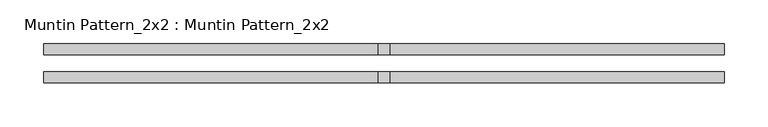
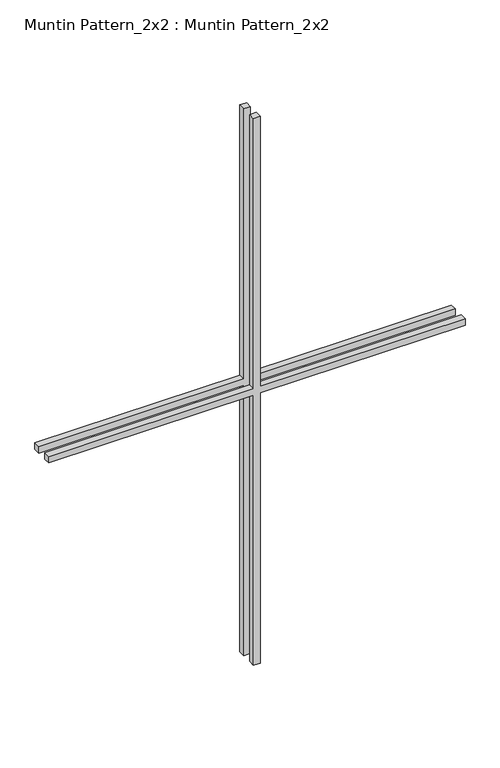
"""IFC4 building model written with IfcOpenShell, lengths in millimetres: proxy geometry, Muntin Pattern_2x2 : Muntin Pattern_2x2."""

from ifc_helpers import new_model, si_unit, frame, origin, place, context, project, spatial, polyline, outline, extrude, source, transform, mapped, element, save


def muntin_pattern_2x2_muntin_pattern_2x2_0aa094e9(model_context):
    return source(origin(), model_context, "Body", "SweptSolid", [
        extrude(outline(polyline([(546.1, -6.35), (546.1, -388.9375), (533.4, -388.9375), (533.4, -6.35), (0.0, -6.35), (0.0, 6.35), (533.4, 6.35), (533.4, 388.9375), (546.1, 388.9375), (546.1, 6.35), (1079.5, 6.35), (1079.5, -6.35), (546.1, -6.35)])), frame((0.0, -22.225, 0.0), z_axis=(0.0, 1.0, 0.0), x_axis=(0.0, 0.0, 1.0)), (0.0, 0.0, 1.0), 12.7),
        extrude(outline(polyline([(546.1, -6.35), (546.1, -388.9375), (533.4, -388.9375), (533.4, -6.35), (0.0, -6.35), (0.0, 6.35), (533.4, 6.35), (533.4, 388.9375), (546.1, 388.9375), (546.1, 6.35), (1079.5, 6.35), (1079.5, -6.35), (546.1, -6.35)])), frame((0.0, 9.525, 0.0), z_axis=(0.0, 1.0, 0.0), x_axis=(0.0, 0.0, 1.0)), (0.0, 0.0, 1.0), 12.7),
    ])


if __name__ == "__main__":
    model = new_model("IFC4")
    model_context = context("Model", 3, world=origin())
    ifc_project = project(units=[si_unit("LENGTHUNIT", "METRE", prefix="MILLI")], contexts=[model_context])
    site = spatial("IfcSite", under=ifc_project)
    building = spatial("IfcBuilding", under=site)
    placement = place(None, origin())
    muntin_pattern_2x2_muntin_pattern_2x2_shape = muntin_pattern_2x2_muntin_pattern_2x2_0aa094e9(model_context)
    element("IfcBuildingElementProxy", 1, Name="Muntin Pattern_2x2 : Muntin Pattern_2x2", ObjectType="Muntin Pattern_2x2 : Muntin Pattern_2x2", at=placement, inside=building, context=model_context, shape_type="MappedRepresentation", body=[
        mapped(muntin_pattern_2x2_muntin_pattern_2x2_shape, transform((0.0, 0.0, 0.0), x_axis=(1.0, 0.0, 0.0), y_axis=(0.0, 1.0, 0.0), z_axis=(0.0, 0.0, 1.0))),
    ])
    save(model, "model.ifc")

# Revit data of these elements
# Type "Muntin Pattern_2x2 : Muntin Pattern_2x2"
#   Width [instance default] = 4' - 0"
#   Thickness = 0' - 0 1/2"
#   Height [instance default] = 4' - 0"
#   Distance = 0' - 0 3/4"
#   Interior Material [instance default] = none
#   Exterior Material [instance default] = none
#   Default Elevation = 0
# Element 1 (IfcBuildingElementProxy, "Muntin Pattern_2x2 : Muntin Pattern_2x2")
#   Width = 2' - 6 5/8"
#   Height = 3' - 6 1/2"
#   Interior Material = Wood - Stained
#   Exterior Material = Clad - White
#   Materials on its faces: "Clad - White", "Wood - Stained"
# Materials
#   "Clad - White": class "Wood", colour RGB 242 242 238, transparency 0, Cost = 0
#   "Wood - Stained": class "Wood", colour RGB 224 178 126, transparency 0, Cost = 0
